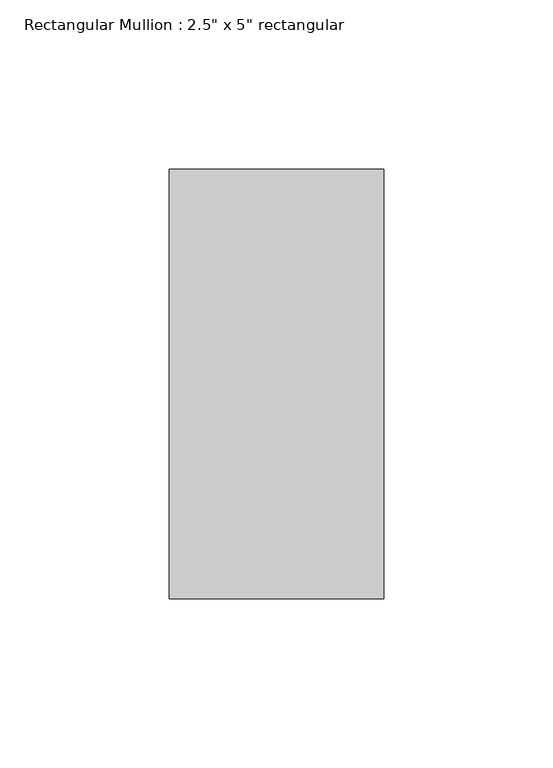
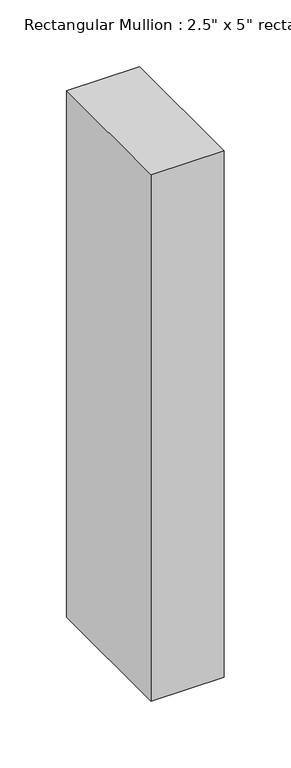
"""IFC4 building model written with IfcOpenShell, lengths in millimetres: member geometry."""

from ifc_helpers import new_model, si_unit, frame, origin, place, context, project, spatial, polyline, outline, extrude, source, transform, mapped, element, save


def member_323df77c(model_context):
    return source(origin(), model_context, "Body", "SweptSolid", [
        extrude(outline(polyline([(31.75, 63.5), (31.75, -63.5), (-31.75, -63.5), (-31.75, 63.5), (31.75, 63.5)])), frame((0.0, 0.0, -482.6), z_axis=(0.0, 0.0, 1.0), x_axis=(1.0, 0.0, 0.0)), (0.0, 0.0, 1.0), 482.6),
    ])


if __name__ == "__main__":
    model = new_model("IFC4")
    model_context = context("Model", 3, world=origin())
    ifc_project = project(units=[si_unit("LENGTHUNIT", "METRE", prefix="MILLI")], contexts=[model_context])
    site = spatial("IfcSite", under=ifc_project)
    building = spatial("IfcBuilding", under=site)
    placement = place(None, origin())
    member_shape = member_323df77c(model_context)
    element("IfcMember", 1, ObjectType="Rectangular Mullion : 2.5\" x 5\" rectangular", at=placement, inside=building, context=model_context, shape_type="MappedRepresentation", body=[
        mapped(member_shape, transform((0.0, 0.0, 0.0), x_axis=(1.0, 0.0, 0.0), y_axis=(0.0, 1.0, 0.0), z_axis=(0.0, 0.0, 1.0))),
    ])
    save(model, "model.ifc")

# Revit data of these elements
# Type "Rectangular Mullion : 2.5\" x 5\" rectangular"
#   built-in parameter 1007304 = 0.416667 (stored number, unit not read)
#   built-in parameter 1007301 = 0.104167 (stored number, unit not read)
#   built-in parameter 1007300 = 0.104167 (stored number, unit not read)
# Element 1 (IfcMember, "Rectangular Mullion : 2.5\" x 5\" rectangular")
#   Materials on its faces: "door colour"
# Materials
#   "door colour": class "Generic", colour RGB 120 120 120, transparency 0, Cost = 0
